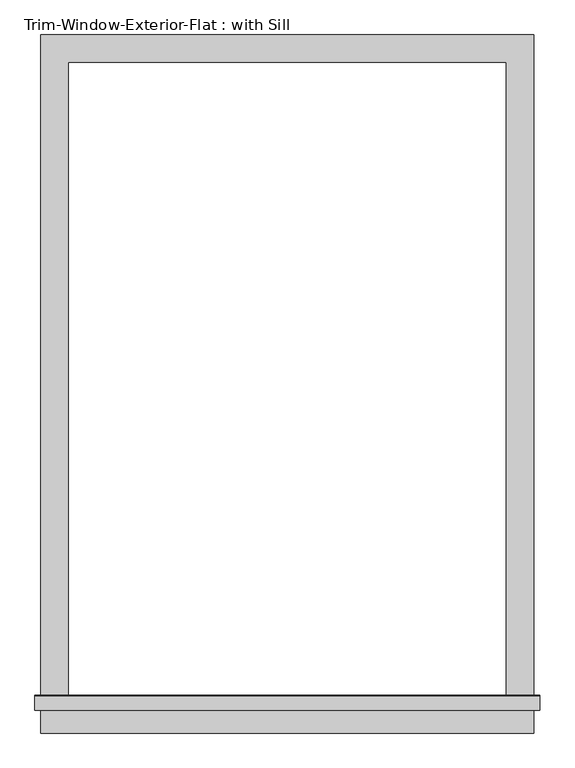
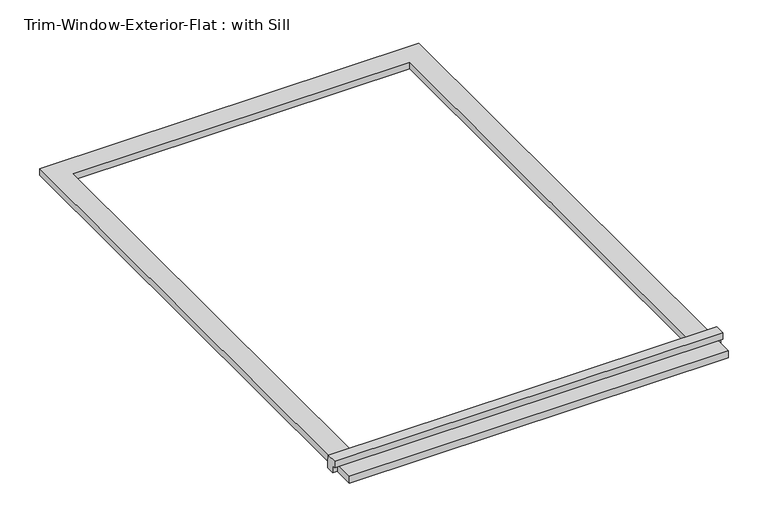
"""IFC4 building model written with IfcOpenShell, lengths in millimetres: proxy geometry, Trim-Window-Exterior-Flat : with Sill."""

from ifc_helpers import new_model, si_unit, frame, origin, origin_with_axes, place, context, project, spatial, polyline, outline, extrude, source, transform, mapped, element, save


def trim_window_exterior_flat_with_sill_fadbc092(model_context):
    return source(origin(), model_context, "Body", "SweptSolid", [
        extrude(outline(polyline([(514.35, -1342.9823709), (514.35, -1400.1323709), (-514.35, -1400.1323709), (-514.35, -1342.9823709), (514.35, -1342.9823709)])), origin_with_axes(), (0.0, 0.0, 1.0), 19.05),
        extrude(outline(polyline([(-1352.55, 38.1), (-1323.2580645, 38.1), (-1320.8, 19.05), (-1320.8, 0.0), (-1342.9823709, 0.0), (-1342.9823709, 19.05), (-1352.55, 19.05), (-1352.55, 38.1)])), frame((-527.05, 0.0, 0.0), z_axis=(1.0, 0.0, 0.0), x_axis=(0.0, 1.0, 0.0)), (0.0, 0.0, 1.0), 1054.1),
        extrude(outline(polyline([(-514.35, 57.15), (514.35, 57.15), (514.35, -1320.8), (457.2, -1320.8), (457.2, 0.0), (-457.2, 0.0), (-457.2, -1320.8), (-514.35, -1320.8), (-514.35, 57.15)])), origin_with_axes(), (0.0, 0.0, 1.0), 19.05),
    ])


if __name__ == "__main__":
    model = new_model("IFC4")
    model_context = context("Model", 3, world=origin())
    ifc_project = project(units=[si_unit("LENGTHUNIT", "METRE", prefix="MILLI")], contexts=[model_context])
    site = spatial("IfcSite", under=ifc_project)
    building = spatial("IfcBuilding", under=site)
    placement = place(None, origin())
    trim_window_exterior_flat_with_sill_shape = trim_window_exterior_flat_with_sill_fadbc092(model_context)
    element("IfcBuildingElementProxy", 1, Name="Trim-Window-Exterior-Flat : with Sill", ObjectType="Trim-Window-Exterior-Flat : with Sill", at=placement, inside=building, context=model_context, shape_type="MappedRepresentation", body=[
        mapped(trim_window_exterior_flat_with_sill_shape, transform((0.0, 0.0, 0.0), x_axis=(1.0, 0.0, 0.0), y_axis=(0.0, 1.0, 0.0), z_axis=(0.0, 0.0, 1.0))),
    ])
    save(model, "model.ifc")

# Revit data of these elements
# Type "Trim-Window-Exterior-Flat : with Sill"
#   Trim Width = 0' - 2 1/4"
#   Trim Thickness_Picture Frame = 0' - 1 1/4"
#   Trim Thickness_with Sill = 0' - 0 3/4"
#   Sill Thickness = 0' - 1 1/4"
#   Opening Width [instance default] = 2' - 0"
#   Opening Height [instance default] = 3' - 0"
#   Default Elevation = 4' - 0"
#   Sill = yes
#   Picture Frame = no
#   Trim Material [instance default] = none
# Element 1 (IfcBuildingElementProxy, "Trim-Window-Exterior-Flat : with Sill")
#   Opening Width = 3' - 0"
#   Opening Height = 4' - 4"
#   Trim Material = Clad - White
#   Materials on its faces: "Clad - White"
# Materials
#   "Clad - White": class "Wood", colour RGB 242 242 238, transparency 0, Cost = 0
